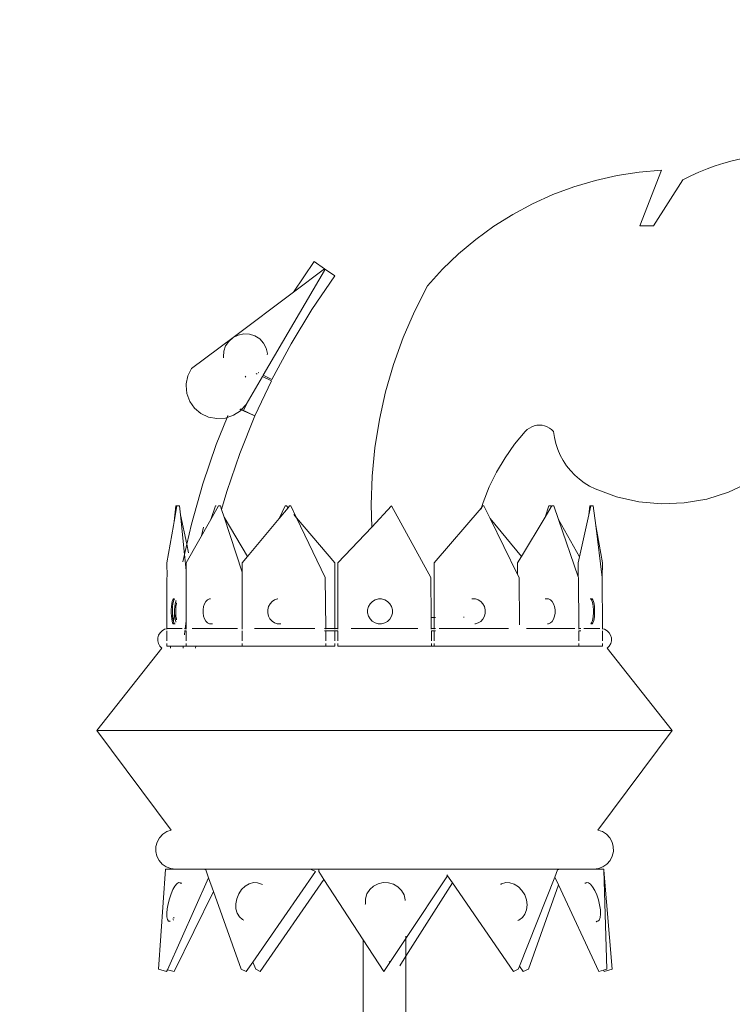
# Model space of a CAD drawing. Units: millimetres. Extents: x 7894 to 8038, y 6851 to 6951.
# Tile 30 of 49: x 7958.696 to 7960.68, y 6925.713 to 6928.453. Entities that reach past the tile are written whole.
import ezdxf

# ---------------------------------------------------------------- set-up
doc = ezdxf.new("R2010")
doc.units = ezdxf.units.MM
doc.layers.add('A-ANNO-DIMS', color=2, linetype='Continuous', lineweight=18)
doc.layers.add('A-FURN-ACCS', color=8, linetype='Continuous', lineweight=13)
doc.styles.get("Standard").update_dxf_attribs({"font": 'arial.ttf'})
doc.dimstyles.new('ISO-25', dxfattribs={"dimtxt": 1, "dimasz": 1, "dimexe": 1.25, "dimexo": 0.625, "dimtad": 1, "dimdec": 0, "dimlunit": 4, "dimtxsty": 'Standard', "dimcen": 2.5, "dimclrt": 1, "dimadec": 0, "dimazin": 0, "dimtfac": 1, "dimtdec": 0, "dimtmove": 0, "dimatfit": 3, "dimfxl": 1, "dimarcsym": 0})

# ---------------------------------------------------------------- blocks, each defined once
blk = doc.blocks.new('DISPLAY-LEAF-FINIAL-Z2_152')
for p, q in [((1.7688, 3.2049, 2.1518), (1.7926, 3.2108, 2.1518)), ((1.5102, 3.1734, 2.1518), (1.5723, 3.1787, 2.1518)), ((1.5723, 3.1787, 2.1518), (1.5113, 3.0242, 2.1518)), ((1.6762, 3.1731, 2.1518), (1.6989, 3.1823, 2.1518)), ((1.6989, 3.1823, 2.1518), (1.7219, 3.1906, 2.1518)), ((1.7219, 3.1906, 2.1518), (1.7452, 3.1982, 2.1518)), ((1.7452, 3.1982, 2.1518), (1.7688, 3.2049, 2.1518)), ((1.3879, 3.1503, 2.1518), (1.4486, 3.1639, 2.1518)), ((1.4486, 3.1639, 2.1518), (1.5102, 3.1734, 2.1518)), ((1.5498, 3.0242, 2.1518), (1.6318, 3.1522, 2.1518)), ((1.6318, 3.1522, 2.1518), (1.6538, 3.163, 2.1518)), ((1.6538, 3.163, 2.1518), (1.6762, 3.1731, 2.1518)), ((1.2698, 3.1109, 2.1518), (1.3281, 3.1326, 2.1518)), ((1.3281, 3.1326, 2.1518), (1.3879, 3.1503, 2.1518)), ((1.213, 3.0852, 2.1518), (1.2698, 3.1109, 2.1518)), ((1.1581, 3.0558, 2.1518), (1.213, 3.0852, 2.1518)), ((1.1053, 3.0227, 2.1518), (1.1581, 3.0558, 2.1518)), ((1.0549, 2.9861, 2.1518), (1.1053, 3.0227, 2.1518)), ((1.5113, 3.0242, 2.1518), (1.5498, 3.0242, 2.1518)), ((1.0071, 2.9462, 2.1518), (1.0549, 2.9861, 2.1518)), ((0.9621, 2.9031, 2.1518), (1.0071, 2.9462, 2.1518)), ((0.6052, 2.9244, 2.1518), (0.5471, 2.8395, 2.1518)), ((0.634, 2.9046, 2.1518), (0.5471, 2.8395, 2.1518)), ((0.634, 2.9046, 2.1518), (0.6052, 2.9244, 2.1518)), ((0.634, 2.9001, 2.1518), (0.634, 2.9046, 2.1518)), ((0.6629, 2.8848, 2.1518), (0.634, 2.9046, 2.1518)), ((0.634, 2.9001, 2.1518), (0.4632, 2.6089, 2.1518)), ((0.5989, 2.7915, 2.1518), (0.6629, 2.8848, 2.1518)), ((0.9202, 2.857, 2.1518), (0.9621, 2.9031, 2.1518)), ((0.9202, 2.857, 2.1518), (0.8844, 2.7861, 2.1518)), ((0.5471, 2.8395, 2.1518), (0.379, 2.7129, 2.1518)), ((0.5406, 2.6956, 2.1518), (0.5989, 2.7915, 2.1518)), ((0.8844, 2.7861, 2.1518), (0.8529, 2.7132, 2.1518)), ((0.379, 2.7129, 2.1518), (0.2637, 2.6275, 2.1518)), ((0.3671, 2.7026, 2.1518), (0.379, 2.7129, 2.1518)), ((0.379, 2.7129, 2.1518), (0.3932, 2.7199, 2.1518)), ((0.3932, 2.7199, 2.1518), (0.4088, 2.7231, 2.1518)), ((0.4088, 2.7231, 2.1518), (0.4248, 2.7223, 2.1518)), ((0.4248, 2.7223, 2.1518), (0.44, 2.7176, 2.1518)), ((0.44, 2.7176, 2.1518), (0.4533, 2.7092, 2.1518)), ((0.8529, 2.7132, 2.1518), (0.8261, 2.6384, 2.1518)), ((0.3535, 2.675, 2.1518), (0.3584, 2.6897, 2.1518)), ((0.3584, 2.6897, 2.1518), (0.3671, 2.7026, 2.1518)), ((0.4533, 2.7092, 2.1518), (0.464, 2.6977, 2.1518)), ((0.464, 2.6977, 2.1518), (0.4713, 2.6839, 2.1518)), ((0.5406, 2.6956, 2.1518), (0.4875, 2.5967, 2.1518)), ((0.3526, 2.6596, 2.1518), (0.3535, 2.675, 2.1518)), ((0.3527, 2.6591, 2.1518), (0.3526, 2.6596, 2.1518)), ((0.3526, 2.6569, 2.1518), (0.3527, 2.6591, 2.1518)), ((0.4713, 2.6839, 2.1518), (0.4746, 2.6689, 2.1518)), ((0.4745, 2.6667, 2.1518), (0.4746, 2.6689, 2.1518)), ((0.4745, 2.6667, 2.1518), (0.4746, 2.6661, 2.1518)), ((0.8261, 2.6384, 2.1518), (0.804, 2.5622, 2.1518)), ((0.2535, 2.6069, 2.1518), (0.249, 2.5845, 2.1518)), ((0.2637, 2.6275, 2.1518), (0.2535, 2.6069, 2.1518)), ((0.4144, 2.6055, 2.1518), (0.4132, 2.6029, 2.1518)), ((0.4608, 2.6047, 2.1518), (0.4152, 2.527, 2.1518)), ((0.4431, 2.613, 2.1518), (0.4459, 2.6117, 2.1518)), ((0.4508, 2.6151, 2.1518), (0.4489, 2.6161, 2.1518)), ((0.4632, 2.6089, 2.1518), (0.4608, 2.6047, 2.1518)), ((0.4858, 2.593, 2.1518), (0.4608, 2.6047, 2.1518)), ((0.4632, 2.6089, 2.1518), (0.4875, 2.5967, 2.1518)), ((0.249, 2.58, 2.1518), (0.249, 2.5845, 2.1518)), ((0.249, 2.58, 2.1518), (0.2508, 2.5572, 2.1518)), ((0.4402, 2.4957, 2.1518), (0.4858, 2.593, 2.1518)), ((0.2508, 2.5572, 2.1518), (0.2586, 2.5356, 2.1518)), ((0.804, 2.5622, 2.1518), (0.7865, 2.4847, 2.1518)), ((0.2586, 2.5356, 2.1518), (0.2719, 2.5167, 2.1518)), ((0.4029, 2.5132, 2.1518), (0.4152, 2.527, 2.1518)), ((0.4202, 2.5355, 2.1518), (0.4085, 2.5106, 2.1518)), ((0.2719, 2.5167, 2.1518), (0.2898, 2.5018, 2.1518)), ((0.2898, 2.5018, 2.1518), (0.3111, 2.4919, 2.1518)), ((0.3628, 2.4909, 2.1518), (0.3802, 2.4968, 2.1518)), ((0.3649, 2.4962, 2.1518), (0.3628, 2.4909, 2.1518)), ((0.3802, 2.4968, 2.1518), (0.3998, 2.5097, 2.1518)), ((0.3978, 2.391, 2.1518), (0.4399, 2.4951, 2.1518)), ((0.3983, 2.5132, 2.1518), (0.4016, 2.5117, 2.1518)), ((0.3998, 2.5097, 2.1518), (0.4016, 2.5117, 2.1518)), ((0.4029, 2.5132, 2.1518), (0.4003, 2.5144, 2.1518)), ((0.4016, 2.5117, 2.1518), (0.4029, 2.5132, 2.1518)), ((0.4016, 2.5117, 2.1518), (0.4399, 2.4951, 2.1518)), ((0.4029, 2.5132, 2.1518), (0.4402, 2.4957, 2.1518)), ((0.4085, 2.5106, 2.1518), (0.4078, 2.509, 2.1518)), ((0.3111, 2.4919, 2.1518), (0.3343, 2.4876, 2.1518)), ((0.3628, 2.4909, 2.1518), (0.3323, 2.4155, 2.1518)), ((0.3343, 2.4876, 2.1518), (0.3579, 2.4893, 2.1518)), ((0.3579, 2.4893, 2.1518), (0.3628, 2.4909, 2.1518)), ((0.7865, 2.4847, 2.1518), (0.774, 2.4062, 2.1518)), ((1.2175, 2.4675, 2.1518), (1.2106, 2.465, 2.1518)), ((1.2247, 2.469, 2.1518), (1.2175, 2.4675, 2.1518)), ((1.2321, 2.4695, 2.1518), (1.2247, 2.469, 2.1518)), ((1.2395, 2.469, 2.1518), (1.2321, 2.4695, 2.1518)), ((1.2467, 2.4675, 2.1518), (1.2395, 2.469, 2.1518)), ((1.2536, 2.465, 2.1518), (1.2467, 2.4675, 2.1518)), ((1.1928, 2.4521, 2.1518), (1.1631, 2.4165, 2.1518)), ((1.1981, 2.4572, 2.1518), (1.1928, 2.4521, 2.1518)), ((1.2041, 2.4615, 2.1518), (1.1981, 2.4572, 2.1518)), ((1.2106, 2.465, 2.1518), (1.2041, 2.4615, 2.1518)), ((1.2601, 2.4615, 2.1518), (1.2536, 2.465, 2.1518)), ((1.2661, 2.4572, 2.1518), (1.2601, 2.4615, 2.1518)), ((1.2714, 2.4521, 2.1518), (1.2661, 2.4572, 2.1518)), ((1.274, 2.435, 2.1518), (1.2714, 2.4521, 2.1518)), ((0.3323, 2.4155, 2.1518), (0.2946, 2.3057, 2.1518)), ((1.1631, 2.4165, 2.1518), (1.1364, 2.3788, 2.1518)), ((1.278, 2.4183, 2.1518), (1.274, 2.435, 2.1518)), ((1.2834, 2.4019, 2.1518), (1.278, 2.4183, 2.1518)), ((0.3614, 2.2848, 2.1518), (0.3978, 2.391, 2.1518)), ((0.774, 2.4062, 2.1518), (0.7662, 2.3272, 2.1518)), ((1.2903, 2.3861, 2.1518), (1.2834, 2.4019, 2.1518)), ((1.2985, 2.371, 2.1518), (1.2903, 2.3861, 2.1518)), ((1.1364, 2.3788, 2.1518), (1.1127, 2.339, 2.1518)), ((1.308, 2.3566, 2.1518), (1.2985, 2.371, 2.1518)), ((1.3187, 2.3431, 2.1518), (1.308, 2.3566, 2.1518)), ((1.1127, 2.339, 2.1518), (1.0923, 2.2975, 2.1518)), ((1.3305, 2.3306, 2.1518), (1.3187, 2.3431, 2.1518)), ((1.3434, 2.3192, 2.1518), (1.3305, 2.3306, 2.1518)), ((0.2946, 2.3057, 2.1518), (0.263, 2.1941, 2.1518)), ((0.7662, 2.3272, 2.1518), (0.7634, 2.2478, 2.1518)), ((1.3572, 2.3089, 2.1518), (1.3434, 2.3192, 2.1518)), ((1.3719, 2.2999, 2.1518), (1.3572, 2.3089, 2.1518)), ((1.8161, 2.3099, 2.1518), (1.7585, 2.283, 2.1518)), ((0.3472, 2.2349, 2.1518), (0.3614, 2.2848, 2.1518)), ((1.0923, 2.2975, 2.1518), (1.0752, 2.2545, 2.1518)), ((1.3873, 2.2921, 2.1518), (1.3719, 2.2999, 2.1518)), ((1.4468, 2.2701, 2.1518), (1.3873, 2.2921, 2.1518)), ((1.7585, 2.283, 2.1518), (1.698, 2.2639, 2.1518)), ((0.7634, 2.2478, 2.1518), (0.7651, 2.1857, 2.1518)), ((1.0752, 2.2545, 2.1518), (1.0707, 2.2401, 2.1518)), ((1.5088, 2.256, 2.1518), (1.4468, 2.2701, 2.1518)), ((1.572, 2.2503, 2.1518), (1.5088, 2.256, 2.1518)), ((1.6354, 2.2529, 2.1518), (1.572, 2.2503, 2.1518)), ((1.698, 2.2639, 2.1518), (1.6354, 2.2529, 2.1518)), ((0.2147, 2.201, 2.1518), (0.2202, 2.2445, 2.1518)), ((0.223, 2.2445, 2.1518), (0.2147, 2.201, 2.1518)), ((0.223, 2.2445, 2.1518), (0.2202, 2.2445, 2.1518)), ((0.223, 2.2445, 2.1518), (0.2299, 2.2445, 2.1518)), ((0.2325, 2.2195, 2.1518), (0.2299, 2.2445, 2.1518)), ((0.2325, 2.2195, 2.1518), (0.2504, 2.1381, 2.1518)), ((0.2439, 2.1095, 2.1518), (0.2325, 2.2195, 2.1518)), ((0.3171, 2.2068, 2.1518), (0.3302, 2.2445, 2.1518)), ((0.3384, 2.2445, 2.1518), (0.3171, 2.2068, 2.1518)), ((0.3318, 2.2445, 2.1518), (0.3302, 2.2445, 2.1518)), ((0.344, 2.2445, 2.1518), (0.3384, 2.2445, 2.1518)), ((0.3472, 2.2349, 2.1518), (0.344, 2.2445, 2.1518)), ((0.3543, 2.2133, 2.1518), (0.3472, 2.2349, 2.1518)), ((0.5072, 2.2093, 2.1518), (0.5246, 2.2445, 2.1518)), ((0.5322, 2.2392, 2.1518), (0.5072, 2.2093, 2.1518)), ((0.5277, 2.2445, 2.1518), (0.5246, 2.2445, 2.1518)), ((0.5277, 2.2445, 2.1518), (0.5322, 2.2392, 2.1518)), ((0.5366, 2.2445, 2.1518), (0.5322, 2.2392, 2.1518)), ((0.5399, 2.2445, 2.1518), (0.5366, 2.2445, 2.1518)), ((0.5559, 2.2114, 2.1518), (0.5399, 2.2445, 2.1518)), ((0.5482, 2.2204, 2.1518), (0.5559, 2.2114, 2.1518)), ((0.8207, 2.2445, 2.1518), (0.7651, 2.1857, 2.1518)), ((0.93, 2.0453, 2.1518), (0.8207, 2.2445, 2.1518)), ((1.0703, 2.2388, 2.1518), (0.9393, 2.0859, 2.1518)), ((1.0703, 2.2388, 2.1518), (1.069, 2.2345, 2.1518)), ((1.0707, 2.2401, 2.1518), (1.0703, 2.2388, 2.1518)), ((1.0703, 2.2388, 2.1518), (1.0715, 2.2374, 2.1518)), ((1.0745, 2.2445, 2.1518), (1.0707, 2.2401, 2.1518)), ((1.0745, 2.2445, 2.1518), (1.0775, 2.2445, 2.1518)), ((1.0949, 2.2093, 2.1518), (1.0775, 2.2445, 2.1518)), ((1.2478, 2.2133, 2.1518), (1.2581, 2.2445, 2.1518)), ((1.2651, 2.2421, 2.1518), (1.2478, 2.2133, 2.1518)), ((1.2581, 2.2445, 2.1518), (1.2637, 2.2445, 2.1518)), ((1.2637, 2.2445, 2.1518), (1.2651, 2.2421, 2.1518)), ((1.2666, 2.2445, 2.1518), (1.2651, 2.2421, 2.1518)), ((1.2666, 2.2445, 2.1518), (1.272, 2.2445, 2.1518)), ((1.2851, 2.2068, 2.1518), (1.272, 2.2445, 2.1518)), ((1.3696, 2.2195, 2.1518), (1.344, 2.1028, 2.1518)), ((1.3696, 2.2195, 2.1518), (1.3722, 2.2445, 2.1518)), ((1.3751, 2.2445, 2.1518), (1.3696, 2.2195, 2.1518)), ((1.3722, 2.2445, 2.1518), (1.3751, 2.2445, 2.1518)), ((1.3751, 2.2445, 2.1518), (1.3819, 2.2445, 2.1518)), ((1.3819, 2.2445, 2.1518), (1.3889, 2.1901, 2.1518)), ((0.2133, 2.1901, 2.1518), (0.2147, 2.201, 2.1518)), ((0.3171, 2.2068, 2.1518), (0.2485, 2.0859, 2.1518)), ((0.263, 2.1941, 2.1518), (0.2504, 2.1381, 2.1518)), ((0.3543, 2.2133, 2.1518), (0.4197, 2.1042, 2.1518)), ((0.4044, 2.0607, 2.1518), (0.3543, 2.2133, 2.1518)), ((0.5072, 2.2093, 2.1518), (0.4197, 2.1042, 2.1518)), ((0.5559, 2.2114, 2.1518), (0.6628, 2.0859, 2.1518)), ((0.636, 2.0453, 2.1518), (0.5559, 2.2114, 2.1518)), ((1.0949, 2.2093, 2.1518), (1.1824, 2.1042, 2.1518)), ((1.0949, 2.2093, 2.1518), (1.1714, 2.0542, 2.1518)), ((1.2478, 2.2133, 2.1518), (1.1824, 2.1042, 2.1518)), ((1.2851, 2.2068, 2.1518), (1.344, 2.1028, 2.1518)), ((1.2851, 2.2068, 2.1518), (1.3403, 2.0478, 2.1518)), ((0.2133, 2.1901, 2.1518), (0.1946, 2.0859, 2.1518)), ((0.2969, 2.1855, 2.1518), (0.2915, 2.1618, 2.1518)), ((0.7651, 2.1857, 2.1518), (0.6705, 2.0859, 2.1518)), ((1.3889, 2.1901, 2.1518), (1.4075, 2.0859, 2.1518)), ((1.4073, 2.0453, 2.1518), (1.3889, 2.1901, 2.1518)), ((0.2504, 2.1381, 2.1518), (0.2439, 2.1095, 2.1518)), ((0.2504, 2.1381, 2.1518), (0.2555, 2.1145, 2.1518)), ((0.1946, 2.0859, 2.1518), (0.1952, 2.0478, 2.1518)), ((0.2439, 2.1095, 2.1518), (0.2392, 2.0887, 2.1518)), ((0.2485, 2.0654, 2.1518), (0.2439, 2.1095, 2.1518)), ((0.2485, 2.0859, 2.1518), (0.2485, 2.0654, 2.1518)), ((0.4197, 2.1042, 2.1518), (0.4044, 2.0859, 2.1518)), ((0.4044, 2.0859, 2.1518), (0.4044, 2.0607, 2.1518)), ((0.6628, 2.0859, 2.1518), (0.6628, 1.9035, 2.1518)), ((0.6705, 2.0859, 2.1518), (0.6705, 1.9035, 2.1518)), ((0.9393, 2.0859, 2.1518), (0.9393, 1.9343, 2.1518)), ((1.1824, 2.1042, 2.1518), (1.1714, 2.0859, 2.1518)), ((1.1714, 2.0859, 2.1518), (1.1714, 2.0542, 2.1518)), ((1.344, 2.1028, 2.1518), (1.3403, 2.0859, 2.1518)), ((1.3403, 2.0859, 2.1518), (1.3403, 2.0478, 2.1518)), ((1.4075, 2.0859, 2.1518), (1.4073, 2.0453, 2.1518)), ((0.2485, 2.0654, 2.1518), (0.2485, 1.9035, 2.1518)), ((0.4044, 2.0607, 2.1518), (0.4044, 1.9015, 2.1518)), ((0.1949, 2.0453, 2.1518), (0.1946, 1.903, 2.1518)), ((0.1949, 2.0453, 2.1518), (0.1952, 2.0478, 2.1518)), ((0.636, 2.0453, 2.1518), (0.6371, 1.9035, 2.1518)), ((0.93, 2.0453, 2.1518), (0.9309, 1.9342, 2.1518)), ((1.1758, 2.0453, 2.1518), (1.1714, 2.0542, 2.1518)), ((1.1758, 2.0453, 2.1518), (1.1768, 1.9142, 2.1518)), ((1.3412, 2.0453, 2.1518), (1.3403, 2.0478, 2.1518)), ((1.3412, 2.0453, 2.1518), (1.3419, 1.9035, 2.1518)), ((1.4073, 2.0453, 2.1518), (1.4075, 1.903, 2.1518)), ((0.2074, 1.9648, 2.1518), (0.2082, 1.9727, 2.1518)), ((0.2082, 1.9727, 2.1518), (0.2095, 1.9791, 2.1518)), ((0.2095, 1.9791, 2.1518), (0.211, 1.9837, 2.1518)), ((0.2108, 1.9648, 2.1518), (0.2117, 1.9727, 2.1518)), ((0.211, 1.9837, 2.1518), (0.2126, 1.986, 2.1518)), ((0.2117, 1.9727, 2.1518), (0.2129, 1.9791, 2.1518)), ((0.2161, 1.986, 2.1518), (0.2126, 1.986, 2.1518)), ((0.2129, 1.9791, 2.1518), (0.2144, 1.9837, 2.1518)), ((0.2144, 1.9837, 2.1518), (0.2161, 1.986, 2.1518)), ((0.2194, 1.979, 2.1518), (0.2179, 1.9725, 2.1518)), ((0.2202, 1.9812, 2.1518), (0.2194, 1.979, 2.1518)), ((0.2204, 1.9806, 2.1518), (0.2194, 1.979, 2.1518)), ((0.2218, 1.9746, 2.1518), (0.2213, 1.9725, 2.1518)), ((0.2969, 1.9648, 2.1518), (0.2996, 1.9727, 2.1518)), ((0.2996, 1.9727, 2.1518), (0.3035, 1.9791, 2.1518)), ((0.3035, 1.9791, 2.1518), (0.3083, 1.9837, 2.1518)), ((0.3083, 1.9837, 2.1518), (0.3135, 1.986, 2.1518)), ((0.3163, 1.986, 2.1518), (0.3135, 1.986, 2.1518)), ((0.478, 1.9648, 2.1518), (0.482, 1.9727, 2.1518)), ((0.482, 1.9727, 2.1518), (0.4877, 1.9791, 2.1518)), ((0.4877, 1.9791, 2.1518), (0.4947, 1.9837, 2.1518)), ((0.4947, 1.9837, 2.1518), (0.5025, 1.986, 2.1518)), ((0.5041, 1.986, 2.1518), (0.5025, 1.986, 2.1518)), ((0.756, 1.9648, 2.1518), (0.7606, 1.9727, 2.1518)), ((0.7606, 1.9727, 2.1518), (0.7671, 1.9791, 2.1518)), ((0.7671, 1.9791, 2.1518), (0.775, 1.9837, 2.1518)), ((0.775, 1.9837, 2.1518), (0.7838, 1.986, 2.1518)), ((0.7838, 1.986, 2.1518), (0.7929, 1.986, 2.1518)), ((0.7929, 1.986, 2.1518), (0.8018, 1.9836, 2.1518)), ((0.8018, 1.9836, 2.1518), (0.8096, 1.979, 2.1518)), ((0.8096, 1.979, 2.1518), (0.8161, 1.9725, 2.1518)), ((1.0443, 1.986, 2.1518), (1.0459, 1.986, 2.1518)), ((1.0459, 1.986, 2.1518), (1.0541, 1.986, 2.1518)), ((1.0541, 1.986, 2.1518), (1.062, 1.9836, 2.1518)), ((1.062, 1.9836, 2.1518), (1.0691, 1.979, 2.1518)), ((1.0691, 1.979, 2.1518), (1.0749, 1.9725, 2.1518)), ((1.2486, 1.986, 2.1518), (1.2513, 1.986, 2.1518)), ((1.2513, 1.986, 2.1518), (1.2571, 1.986, 2.1518)), ((1.2571, 1.986, 2.1518), (1.2627, 1.9836, 2.1518)), ((1.2627, 1.9836, 2.1518), (1.2677, 1.979, 2.1518)), ((1.2677, 1.979, 2.1518), (1.2717, 1.9725, 2.1518)), ((1.3734, 1.986, 2.1518), (1.3755, 1.986, 2.1518)), ((1.3755, 1.986, 2.1518), (1.3775, 1.9836, 2.1518)), ((1.3755, 1.986, 2.1518), (1.3768, 1.986, 2.1518)), ((1.3768, 1.986, 2.1518), (1.3789, 1.986, 2.1518)), ((1.3775, 1.9836, 2.1518), (1.3794, 1.979, 2.1518)), ((1.3789, 1.986, 2.1518), (1.3809, 1.9836, 2.1518)), ((1.3794, 1.979, 2.1518), (1.3809, 1.9725, 2.1518)), ((1.3809, 1.9836, 2.1518), (1.3828, 1.979, 2.1518)), ((1.3828, 1.979, 2.1518), (1.3843, 1.9725, 2.1518)), ((0.2069, 1.956, 2.1518), (0.2074, 1.9648, 2.1518)), ((0.2069, 1.9469, 2.1518), (0.2069, 1.956, 2.1518)), ((0.2073, 1.938, 2.1518), (0.2069, 1.9469, 2.1518)), ((0.2103, 1.956, 2.1518), (0.2108, 1.9648, 2.1518)), ((0.2103, 1.9469, 2.1518), (0.2103, 1.956, 2.1518)), ((0.2108, 1.938, 2.1518), (0.2103, 1.9469, 2.1518)), ((0.2163, 1.9467, 2.1518), (0.2129, 1.9237, 2.1518)), ((0.2168, 1.9646, 2.1518), (0.2163, 1.9558, 2.1518)), ((0.2163, 1.9558, 2.1518), (0.2163, 1.9467, 2.1518)), ((0.2163, 1.9467, 2.1518), (0.2168, 1.9379, 2.1518)), ((0.2179, 1.9725, 2.1518), (0.2168, 1.9646, 2.1518)), ((0.218, 1.9665, 2.1518), (0.2168, 1.9646, 2.1518)), ((0.2179, 1.9725, 2.1518), (0.218, 1.9665, 2.1518)), ((0.2202, 1.9646, 2.1518), (0.2197, 1.9558, 2.1518)), ((0.2197, 1.9558, 2.1518), (0.2197, 1.9467, 2.1518)), ((0.2197, 1.9467, 2.1518), (0.2202, 1.9379, 2.1518)), ((0.2213, 1.9725, 2.1518), (0.2202, 1.9646, 2.1518)), ((0.2955, 1.956, 2.1518), (0.2969, 1.9648, 2.1518)), ((0.2955, 1.9469, 2.1518), (0.2955, 1.956, 2.1518)), ((0.2969, 1.938, 2.1518), (0.2955, 1.9469, 2.1518)), ((0.4759, 1.956, 2.1518), (0.478, 1.9648, 2.1518)), ((0.4759, 1.9469, 2.1518), (0.4759, 1.956, 2.1518)), ((0.4779, 1.938, 2.1518), (0.4759, 1.9469, 2.1518)), ((0.7536, 1.956, 2.1518), (0.756, 1.9648, 2.1518)), ((0.7536, 1.9469, 2.1518), (0.7536, 1.956, 2.1518)), ((0.756, 1.938, 2.1518), (0.7536, 1.9469, 2.1518)), ((0.8161, 1.9725, 2.1518), (0.8206, 1.9646, 2.1518)), ((0.8229, 1.9467, 2.1518), (0.8205, 1.9379, 2.1518)), ((0.8206, 1.9646, 2.1518), (0.823, 1.9558, 2.1518)), ((0.823, 1.9558, 2.1518), (0.8229, 1.9467, 2.1518)), ((1.0749, 1.9725, 2.1518), (1.079, 1.9646, 2.1518)), ((1.081, 1.9467, 2.1518), (1.0789, 1.9379, 2.1518)), ((1.079, 1.9646, 2.1518), (1.0811, 1.9558, 2.1518)), ((1.0811, 1.9558, 2.1518), (1.081, 1.9467, 2.1518)), ((1.2717, 1.9725, 2.1518), (1.2746, 1.9646, 2.1518)), ((1.2746, 1.9646, 2.1518), (1.2761, 1.9558, 2.1518)), ((1.2761, 1.9467, 2.1518), (1.2746, 1.9379, 2.1518)), ((1.2761, 1.9558, 2.1518), (1.2761, 1.9467, 2.1518)), ((1.3809, 1.9725, 2.1518), (1.3819, 1.9646, 2.1518)), ((1.3819, 1.9646, 2.1518), (1.3825, 1.9558, 2.1518)), ((1.3824, 1.9467, 2.1518), (1.3819, 1.9379, 2.1518)), ((1.3825, 1.9558, 2.1518), (1.3824, 1.9467, 2.1518)), ((1.3843, 1.9725, 2.1518), (1.3853, 1.9646, 2.1518)), ((1.3853, 1.9646, 2.1518), (1.3859, 1.9558, 2.1518)), ((1.3858, 1.9467, 2.1518), (1.3853, 1.9379, 2.1518)), ((1.3859, 1.9558, 2.1518), (1.3858, 1.9467, 2.1518)), ((0.2082, 1.9301, 2.1518), (0.2073, 1.938, 2.1518)), ((0.2094, 1.9237, 2.1518), (0.2082, 1.9301, 2.1518)), ((0.2109, 1.9191, 2.1518), (0.2094, 1.9237, 2.1518)), ((0.2116, 1.9301, 2.1518), (0.2108, 1.938, 2.1518)), ((0.2126, 1.9167, 2.1518), (0.2109, 1.9191, 2.1518)), ((0.2129, 1.9237, 2.1518), (0.2116, 1.9301, 2.1518)), ((0.2143, 1.9191, 2.1518), (0.2129, 1.9237, 2.1518)), ((0.216, 1.9167, 2.1518), (0.2143, 1.9191, 2.1518)), ((0.2168, 1.9379, 2.1518), (0.2179, 1.93, 2.1518)), ((0.2179, 1.93, 2.1518), (0.2194, 1.9235, 2.1518)), ((0.2194, 1.9235, 2.1518), (0.2202, 1.9215, 2.1518)), ((0.2202, 1.9379, 2.1518), (0.2213, 1.93, 2.1518)), ((0.2213, 1.93, 2.1518), (0.2218, 1.928, 2.1518)), ((0.2485, 1.9251, 2.1518), (0.2458, 1.9015, 2.1518)), ((0.2996, 1.9301, 2.1518), (0.2969, 1.938, 2.1518)), ((0.3034, 1.9237, 2.1518), (0.2996, 1.9301, 2.1518)), ((0.3082, 1.9191, 2.1518), (0.3034, 1.9237, 2.1518)), ((0.3134, 1.9167, 2.1518), (0.3082, 1.9191, 2.1518)), ((0.4819, 1.9301, 2.1518), (0.4779, 1.938, 2.1518)), ((0.4876, 1.9237, 2.1518), (0.4819, 1.9301, 2.1518)), ((0.4945, 1.9191, 2.1518), (0.4876, 1.9237, 2.1518)), ((0.5023, 1.9167, 2.1518), (0.4945, 1.9191, 2.1518)), ((0.7605, 1.9301, 2.1518), (0.756, 1.938, 2.1518)), ((0.7669, 1.9237, 2.1518), (0.7605, 1.9301, 2.1518)), ((0.7748, 1.9191, 2.1518), (0.7669, 1.9237, 2.1518)), ((0.7836, 1.9167, 2.1518), (0.7748, 1.9191, 2.1518)), ((0.8016, 1.919, 2.1518), (0.7928, 1.9167, 2.1518)), ((0.8095, 1.9235, 2.1518), (0.8016, 1.919, 2.1518)), ((0.816, 1.93, 2.1518), (0.8095, 1.9235, 2.1518)), ((0.8205, 1.9379, 2.1518), (0.816, 1.93, 2.1518)), ((0.9393, 1.9343, 2.1518), (0.9309, 1.9342, 2.1518)), ((0.9309, 1.9342, 2.1518), (0.9312, 1.9035, 2.1518)), ((0.9424, 1.9343, 2.1518), (0.9393, 1.9343, 2.1518)), ((0.9393, 1.9343, 2.1518), (0.9393, 1.9035, 2.1518)), ((1.0224, 1.935, 2.1518), (1.0208, 1.935, 2.1518)), ((1.0618, 1.919, 2.1518), (1.0539, 1.9167, 2.1518)), ((1.069, 1.9235, 2.1518), (1.0618, 1.919, 2.1518)), ((1.0748, 1.93, 2.1518), (1.069, 1.9235, 2.1518)), ((1.0789, 1.9379, 2.1518), (1.0748, 1.93, 2.1518)), ((1.2626, 1.919, 2.1518), (1.257, 1.9167, 2.1518)), ((1.2676, 1.9235, 2.1518), (1.2626, 1.919, 2.1518)), ((1.2717, 1.93, 2.1518), (1.2676, 1.9235, 2.1518)), ((1.2746, 1.9379, 2.1518), (1.2717, 1.93, 2.1518)), ((1.3775, 1.919, 2.1518), (1.3755, 1.9167, 2.1518)), ((1.3793, 1.9235, 2.1518), (1.3775, 1.919, 2.1518)), ((1.3809, 1.919, 2.1518), (1.3789, 1.9167, 2.1518)), ((1.3808, 1.93, 2.1518), (1.3793, 1.9235, 2.1518)), ((1.3819, 1.9379, 2.1518), (1.3808, 1.93, 2.1518)), ((1.3827, 1.9235, 2.1518), (1.3809, 1.919, 2.1518)), ((1.3842, 1.93, 2.1518), (1.3827, 1.9235, 2.1518)), ((1.3853, 1.9379, 2.1518), (1.3842, 1.93, 2.1518)), ((0.1719, 1.8852, 2.1518), (0.1759, 1.892, 2.1518)), ((0.1759, 1.892, 2.1518), (0.1817, 1.8976, 2.1518)), ((0.1817, 1.8976, 2.1518), (0.1886, 1.9015, 2.1518)), ((0.1886, 1.9015, 2.1518), (0.1946, 1.903, 2.1518)), ((0.1946, 1.8976, 2.1518), (0.1945, 1.8695, 2.1518)), ((0.1946, 1.903, 2.1518), (0.1964, 1.9035, 2.1518)), ((0.1946, 1.903, 2.1518), (0.1946, 1.9015, 2.1518)), ((0.1964, 1.9035, 2.1518), (0.1977, 1.9034, 2.1518)), ((0.1964, 1.9035, 2.1518), (0.1969, 1.9035, 2.1518)), ((0.2373, 1.9035, 2.1518), (0.1977, 1.9034, 2.1518)), ((0.2143, 1.9167, 2.1518), (0.2126, 1.9167, 2.1518)), ((0.216, 1.9167, 2.1518), (0.2143, 1.9167, 2.1518)), ((0.2177, 1.9167, 2.1518), (0.216, 1.9167, 2.1518)), ((0.2485, 1.9035, 2.1518), (0.2439, 1.9035, 2.1518)), ((0.2453, 1.8976, 2.1518), (0.2439, 1.8856, 2.1518)), ((0.2485, 1.8971, 2.1518), (0.2439, 1.8971, 2.1518)), ((0.2485, 1.9035, 2.1518), (0.2485, 1.9015, 2.1518)), ((0.2485, 1.8976, 2.1518), (0.2485, 1.8971, 2.1518)), ((0.2485, 1.8971, 2.1518), (0.2485, 1.8695, 2.1518)), ((0.3912, 1.9035, 2.1518), (0.265, 1.9035, 2.1518)), ((0.3189, 1.9167, 2.1518), (0.3134, 1.9167, 2.1518)), ((0.3217, 1.9167, 2.1518), (0.3189, 1.9167, 2.1518)), ((0.4044, 1.8976, 2.1518), (0.4044, 1.8695, 2.1518)), ((0.4385, 1.9035, 2.1518), (0.6066, 1.9035, 2.1518)), ((0.5103, 1.9167, 2.1518), (0.5023, 1.9167, 2.1518)), ((0.512, 1.9167, 2.1518), (0.5103, 1.9167, 2.1518)), ((0.6371, 1.9035, 2.1518), (0.6338, 1.9035, 2.1518)), ((0.6371, 1.8971, 2.1518), (0.6338, 1.8971, 2.1518)), ((0.6371, 1.9035, 2.1518), (0.6371, 1.9015, 2.1518)), ((0.6628, 1.9035, 2.1518), (0.6371, 1.9035, 2.1518)), ((0.6371, 1.8976, 2.1518), (0.6371, 1.8971, 2.1518)), ((0.6371, 1.8971, 2.1518), (0.6373, 1.8695, 2.1518)), ((0.6628, 1.8971, 2.1518), (0.6371, 1.8971, 2.1518)), ((0.6628, 1.9035, 2.1518), (0.6705, 1.9035, 2.1518)), ((0.6628, 1.9035, 2.1518), (0.6628, 1.9015, 2.1518)), ((0.6628, 1.8976, 2.1518), (0.6628, 1.8971, 2.1518)), ((0.6628, 1.8971, 2.1518), (0.6628, 1.8695, 2.1518)), ((0.6705, 1.8971, 2.1518), (0.6628, 1.8971, 2.1518)), ((0.6705, 1.9035, 2.1518), (0.6705, 1.9015, 2.1518)), ((0.6705, 1.8976, 2.1518), (0.6705, 1.8971, 2.1518)), ((0.6705, 1.8971, 2.1518), (0.6705, 1.8695, 2.1518)), ((0.7081, 1.9035, 2.1518), (0.894, 1.9035, 2.1518)), ((0.7928, 1.9167, 2.1518), (0.7836, 1.9167, 2.1518)), ((0.9312, 1.9035, 2.1518), (0.9312, 1.9015, 2.1518)), ((0.9393, 1.9035, 2.1518), (0.9312, 1.9035, 2.1518)), ((0.9313, 1.8976, 2.1518), (0.9313, 1.8971, 2.1518)), ((0.9313, 1.8971, 2.1518), (0.9315, 1.8695, 2.1518)), ((0.9393, 1.8971, 2.1518), (0.9313, 1.8971, 2.1518)), ((0.9424, 1.9035, 2.1518), (0.9393, 1.9035, 2.1518)), ((0.9393, 1.9035, 2.1518), (0.9393, 1.9015, 2.1518)), ((0.9393, 1.8976, 2.1518), (0.9393, 1.8971, 2.1518)), ((0.9424, 1.8971, 2.1518), (0.9393, 1.8971, 2.1518)), ((0.9393, 1.8971, 2.1518), (0.9393, 1.8695, 2.1518)), ((0.9534, 1.9035, 2.1518), (1.1456, 1.9035, 2.1518)), ((1.0524, 1.9167, 2.1518), (1.0539, 1.9167, 2.1518)), ((1.3304, 1.9035, 2.1518), (1.1965, 1.9035, 2.1518)), ((1.2543, 1.9167, 2.1518), (1.257, 1.9167, 2.1518)), ((1.3471, 1.9035, 2.1518), (1.3419, 1.9035, 2.1518)), ((1.3419, 1.9035, 2.1518), (1.342, 1.9015, 2.1518)), ((1.342, 1.8976, 2.1518), (1.342, 1.8971, 2.1518)), ((1.3471, 1.8971, 2.1518), (1.342, 1.8971, 2.1518)), ((1.342, 1.8971, 2.1518), (1.3421, 1.8695, 2.1518)), ((1.3561, 1.9035, 2.1518), (1.4004, 1.9035, 2.1518)), ((1.3755, 1.9167, 2.1518), (1.3789, 1.9167, 2.1518)), ((1.4075, 1.903, 2.1518), (1.4135, 1.9015, 2.1518)), ((1.4075, 1.903, 2.1518), (1.4075, 1.9015, 2.1518)), ((1.4075, 1.8976, 2.1518), (1.4075, 1.8695, 2.1518)), ((1.4135, 1.9015, 2.1518), (1.4205, 1.8976, 2.1518)), ((1.4205, 1.8976, 2.1518), (1.4262, 1.892, 2.1518)), ((1.4262, 1.892, 2.1518), (1.4303, 1.8852, 2.1518)), ((0.1696, 1.8695, 2.1518), (0.1697, 1.8775, 2.1518)), ((0.1715, 1.8618, 2.1518), (0.1696, 1.8695, 2.1518)), ((0.1697, 1.8775, 2.1518), (0.1719, 1.8852, 2.1518)), ((1.4303, 1.8852, 2.1518), (1.4325, 1.8775, 2.1518)), ((1.4326, 1.8695, 2.1518), (1.4306, 1.8618, 2.1518)), ((1.4325, 1.8775, 2.1518), (1.4326, 1.8695, 2.1518)), ((0, 1.6201, 2.1518), (0.181, 1.8491, 2.1518)), ((0.1754, 1.8548, 2.1518), (0.1715, 1.8618, 2.1518)), ((0.181, 1.8491, 2.1518), (0.1754, 1.8548, 2.1518)), ((0.1945, 1.8618, 2.1518), (0.1945, 1.8548, 2.1518)), ((0.1952, 1.8548, 2.1518), (0.1945, 1.8548, 2.1518)), ((0.2052, 1.8548, 2.1518), (0.1945, 1.8548, 2.1518)), ((0.2048, 1.8513, 2.1518), (0.2047, 1.8491, 2.1518)), ((0.2052, 1.8548, 2.1518), (0.2048, 1.8513, 2.1518)), ((0.2485, 1.8548, 2.1518), (0.2052, 1.8548, 2.1518)), ((0.2404, 1.8548, 2.1518), (0.2398, 1.8491, 2.1518)), ((0.2485, 1.8618, 2.1518), (0.2485, 1.8548, 2.1518)), ((0.2485, 1.8548, 2.1518), (0.2756, 1.8548, 2.1518)), ((0.2749, 1.8491, 2.1518), (0.2756, 1.8548, 2.1518)), ((0.2756, 1.8548, 2.1518), (0.4049, 1.8548, 2.1518)), ((0.4044, 1.8618, 2.1518), (0.4049, 1.8548, 2.1518)), ((0.4049, 1.8548, 2.1518), (0.6375, 1.8548, 2.1518)), ((0.6374, 1.8618, 2.1518), (0.6375, 1.8548, 2.1518)), ((0.6628, 1.8548, 2.1518), (0.6375, 1.8548, 2.1518)), ((0.6628, 1.8618, 2.1518), (0.6628, 1.8548, 2.1518)), ((0.6705, 1.8618, 2.1518), (0.6705, 1.8548, 2.1518)), ((0.6705, 1.8548, 2.1518), (0.9316, 1.8548, 2.1518)), ((0.9316, 1.8618, 2.1518), (0.9316, 1.8548, 2.1518)), ((0.9393, 1.8548, 2.1518), (0.9316, 1.8548, 2.1518)), ((0.9393, 1.8618, 2.1518), (0.9393, 1.8548, 2.1518)), ((1.3422, 1.8548, 2.1518), (0.9393, 1.8548, 2.1518)), ((1.3422, 1.8618, 2.1518), (1.3422, 1.8548, 2.1518)), ((1.4075, 1.8548, 2.1518), (1.3422, 1.8548, 2.1518)), ((1.4075, 1.8618, 2.1518), (1.4075, 1.8548, 2.1518)), ((1.4267, 1.8548, 2.1518), (1.4212, 1.8491, 2.1518)), ((1.4212, 1.8491, 2.1518), (1.6021, 1.6201, 2.1518)), ((1.4306, 1.8618, 2.1518), (1.4267, 1.8548, 2.1518)), ((0.2072, 1.3429, 2.1518), (0, 1.6201, 2.1518)), ((1.6021, 1.6201, 2.1518), (0, 1.6201, 2.1518)), ((1.6021, 1.6201, 2.1518), (1.395, 1.3429, 2.1518)), ((0.1945, 1.3385, 2.1518), (0.2072, 1.3429, 2.1518)), ((1.395, 1.3429, 2.1518), (1.4076, 1.3385, 2.1518)), ((0.1678, 1.3095, 2.1518), (0.1742, 1.3213, 2.1518)), ((0.1742, 1.3213, 2.1518), (0.1833, 1.3311, 2.1518)), ((0.1833, 1.3311, 2.1518), (0.1945, 1.3385, 2.1518)), ((1.4076, 1.3385, 2.1518), (1.4188, 1.3311, 2.1518)), ((1.4188, 1.3311, 2.1518), (1.4279, 1.3213, 2.1518)), ((1.4279, 1.3213, 2.1518), (1.4344, 1.3095, 2.1518)), ((0.1641, 1.2832, 2.1518), (0.1643, 1.2966, 2.1518)), ((0.1643, 1.2966, 2.1518), (0.1678, 1.3095, 2.1518)), ((1.4344, 1.3095, 2.1518), (1.4378, 1.2966, 2.1518)), ((1.4378, 1.2966, 2.1518), (1.438, 1.2832, 2.1518)), ((0.1672, 1.2701, 2.1518), (0.1641, 1.2832, 2.1518)), ((0.1733, 1.2582, 2.1518), (0.1672, 1.2701, 2.1518)), ((1.435, 1.2701, 2.1518), (1.4288, 1.2582, 2.1518)), ((1.438, 1.2832, 2.1518), (1.435, 1.2701, 2.1518)), ((0.1714, 0.9553, 2.1518), (0.1907, 1.234, 2.1518)), ((0.1821, 1.2481, 2.1518), (0.1733, 1.2582, 2.1518)), ((0.1931, 1.2404, 2.1518), (0.1821, 1.2481, 2.1518)), ((0.2189, 1.234, 2.1518), (0.1907, 1.234, 2.1518)), ((0.2056, 1.2356, 2.1518), (0.1931, 1.2404, 2.1518)), ((0.2189, 1.234, 2.1518), (0.2056, 1.2356, 2.1518)), ((0.2189, 1.234, 2.1518), (0.2969, 1.234, 2.1518)), ((0.2969, 1.234, 2.1518), (0.3022, 1.234, 2.1518)), ((0.3029, 1.2321, 2.1518), (0.2969, 1.234, 2.1518)), ((0.3029, 1.2321, 2.1518), (0.3022, 1.234, 2.1518)), ((0.3022, 1.234, 2.1518), (0.5943, 1.234, 2.1518)), ((0.5943, 1.234, 2.1518), (0.6175, 1.234, 2.1518)), ((0.6087, 1.2276, 2.1518), (0.5943, 1.234, 2.1518)), ((0.6175, 1.2276, 2.1518), (0.6175, 1.234, 2.1518)), ((0.9517, 1.234, 2.1518), (0.6175, 1.234, 2.1518)), ((0.9809, 1.2337, 2.1518), (0.9517, 1.234, 2.1518)), ((0.9809, 1.2337, 2.1518), (0.9815, 1.234, 2.1518)), ((0.9815, 1.234, 2.1518), (0.9829, 1.234, 2.1518)), ((1.2836, 1.234, 2.1518), (0.9829, 1.234, 2.1518)), ((1.2826, 1.2319, 2.1518), (1.2898, 1.234, 2.1518)), ((1.2826, 1.2319, 2.1518), (1.2836, 1.234, 2.1518)), ((1.2836, 1.234, 2.1518), (1.2898, 1.234, 2.1518)), ((1.2898, 1.234, 2.1518), (1.3832, 1.234, 2.1518)), ((1.3965, 1.2356, 2.1518), (1.3832, 1.234, 2.1518)), ((1.41, 1.2337, 2.1518), (1.3832, 1.234, 2.1518)), ((1.409, 1.2404, 2.1518), (1.3965, 1.2356, 2.1518)), ((1.42, 1.2481, 2.1518), (1.409, 1.2404, 2.1518)), ((1.4111, 1.234, 2.1518), (1.41, 1.2337, 2.1518)), ((1.4113, 1.2316, 2.1518), (1.4111, 1.234, 2.1518)), ((1.4288, 1.2582, 2.1518), (1.42, 1.2481, 2.1518)), ((0.1964, 0.9543, 2.1518), (0.3109, 1.2098, 2.1518)), ((0.3109, 1.2098, 2.1518), (0.3029, 1.2321, 2.1518)), ((0.3244, 1.1717, 2.1518), (0.3109, 1.2098, 2.1518)), ((0.4339, 0.9752, 2.1518), (0.6087, 1.2276, 2.1518)), ((0.6322, 1.205, 2.1518), (0.6175, 1.2276, 2.1518)), ((0.8605, 1.0411, 2.1518), (0.9765, 1.2154, 2.1518)), ((0.9765, 1.2154, 2.1518), (0.9744, 1.2185, 2.1518)), ((0.9902, 1.1955, 2.1518), (0.9765, 1.2154, 2.1518)), ((1.1768, 0.964, 2.1518), (1.2748, 1.2121, 2.1518)), ((1.2748, 1.2121, 2.1518), (1.2826, 1.2319, 2.1518)), ((1.285, 1.1903, 2.1518), (1.2748, 1.2121, 2.1518)), ((1.4348, 0.9553, 2.1518), (1.4113, 1.2316, 2.1518)), ((1.4203, 0.9553, 2.1518), (1.4113, 1.2316, 2.1518)), ((0.2118, 1.177, 2.1518), (0.2173, 1.1867, 2.1518)), ((0.2173, 1.1867, 2.1518), (0.2227, 1.1934, 2.1518)), ((0.2227, 1.1934, 2.1518), (0.2276, 1.1967, 2.1518)), ((0.2276, 1.1967, 2.1518), (0.2317, 1.1963, 2.1518)), ((0.2325, 1.1953, 2.1518), (0.2317, 1.1963, 2.1518)), ((0.2325, 1.1953, 2.1518), (0.2366, 1.1949, 2.1518)), ((0.4028, 1.177, 2.1518), (0.4128, 1.1867, 2.1518)), ((0.4128, 1.1867, 2.1518), (0.4241, 1.1934, 2.1518)), ((0.4241, 1.1934, 2.1518), (0.436, 1.1967, 2.1518)), ((0.436, 1.1967, 2.1518), (0.4475, 1.1963, 2.1518)), ((0.4475, 1.1963, 2.1518), (0.4584, 1.192, 2.1518)), ((0.455, 0.949, 2.1518), (0.6322, 1.205, 2.1518)), ((0.4584, 1.192, 2.1518), (0.4611, 1.1909, 2.1518)), ((0.7416, 1.0372, 2.1518), (0.6322, 1.205, 2.1518)), ((0.7597, 1.177, 2.1518), (0.7703, 1.1867, 2.1518)), ((0.7703, 1.1867, 2.1518), (0.7831, 1.1934, 2.1518)), ((0.7831, 1.1934, 2.1518), (0.7973, 1.1967, 2.1518)), ((0.7973, 1.1967, 2.1518), (0.8119, 1.1963, 2.1518)), ((0.8119, 1.1963, 2.1518), (0.8259, 1.1923, 2.1518)), ((0.8259, 1.1923, 2.1518), (0.8383, 1.1849, 2.1518)), ((0.8383, 1.1849, 2.1518), (0.8484, 1.1746, 2.1518)), ((0.8605, 0.9923, 2.1518), (0.9902, 1.1955, 2.1518)), ((1.1599, 0.949, 2.1518), (0.9902, 1.1955, 2.1518)), ((1.1241, 1.1921, 2.1518), (1.1257, 1.1926, 2.1518)), ((1.1257, 1.1926, 2.1518), (1.127, 1.1934, 2.1518)), ((1.127, 1.1934, 2.1518), (1.1382, 1.1967, 2.1518)), ((1.1382, 1.1967, 2.1518), (1.1502, 1.1963, 2.1518)), ((1.1502, 1.1963, 2.1518), (1.1623, 1.1923, 2.1518)), ((1.1623, 1.1923, 2.1518), (1.1737, 1.1849, 2.1518)), ((1.1737, 1.1849, 2.1518), (1.1835, 1.1746, 2.1518)), ((1.2015, 0.9553, 2.1518), (1.285, 1.1903, 2.1518)), ((1.398, 0.949, 2.1518), (1.285, 1.1903, 2.1518)), ((1.359, 1.1953, 2.1518), (1.3638, 1.1967, 2.1518)), ((1.359, 1.1953, 2.1518), (1.3619, 1.1951, 2.1518)), ((1.3638, 1.1967, 2.1518), (1.3687, 1.1963, 2.1518)), ((1.3687, 1.1963, 2.1518), (1.3744, 1.1923, 2.1518)), ((1.3744, 1.1923, 2.1518), (1.3804, 1.1849, 2.1518)), ((1.3804, 1.1849, 2.1518), (1.3863, 1.1746, 2.1518)), ((0.1981, 1.1374, 2.1518), (0.2018, 1.1515, 2.1518)), ((0.2018, 1.1515, 2.1518), (0.2065, 1.165, 2.1518)), ((0.2065, 1.165, 2.1518), (0.2118, 1.177, 2.1518)), ((0.2147, 0.949, 2.1518), (0.3244, 1.1717, 2.1518)), ((0.4015, 0.9553, 2.1518), (0.3244, 1.1717, 2.1518)), ((0.3867, 1.1374, 2.1518), (0.3893, 1.1515, 2.1518)), ((0.3893, 1.1515, 2.1518), (0.3948, 1.165, 2.1518)), ((0.3948, 1.165, 2.1518), (0.4028, 1.177, 2.1518)), ((0.7475, 1.1373, 2.1518), (0.7478, 1.1515, 2.1518)), ((0.7478, 1.1515, 2.1518), (0.752, 1.165, 2.1518)), ((0.752, 1.165, 2.1518), (0.7597, 1.177, 2.1518)), ((0.8484, 1.1746, 2.1518), (0.8553, 1.1622, 2.1518)), ((0.8553, 1.1622, 2.1518), (0.8587, 1.1485, 2.1518)), ((1.1835, 1.1746, 2.1518), (1.1911, 1.1622, 2.1518)), ((1.1911, 1.1622, 2.1518), (1.196, 1.1485, 2.1518)), ((1.3863, 1.1746, 2.1518), (1.3917, 1.1622, 2.1518)), ((1.3917, 1.1622, 2.1518), (1.3963, 1.1485, 2.1518)), ((0.1943, 1.1113, 2.1518), (0.1955, 1.1237, 2.1518)), ((0.1955, 1.1237, 2.1518), (0.1981, 1.1374, 2.1518)), ((0.3871, 1.1237, 2.1518), (0.3867, 1.1374, 2.1518)), ((0.3906, 1.1113, 2.1518), (0.3871, 1.1237, 2.1518)), ((0.7474, 1.1361, 2.1518), (0.7475, 1.1373, 2.1518)), ((0.8587, 1.1471, 2.1518), (0.8587, 1.1485, 2.1518)), ((1.196, 1.1485, 2.1518), (1.1978, 1.1344, 2.1518)), ((1.1978, 1.1344, 2.1518), (1.1964, 1.1209, 2.1518)), ((1.3963, 1.1485, 2.1518), (1.3997, 1.1344, 2.1518)), ((1.3997, 1.1344, 2.1518), (1.4018, 1.1209, 2.1518)), ((0.1946, 1.101, 2.1518), (0.1943, 1.1113, 2.1518)), ((0.1963, 1.0936, 2.1518), (0.1946, 1.101, 2.1518)), ((0.2112, 1.0961, 2.1518), (0.2129, 1.0925, 2.1518)), ((0.2141, 1.1, 2.1518), (0.2145, 1.0978, 2.1518)), ((0.3969, 1.101, 2.1518), (0.3906, 1.1113, 2.1518)), ((0.4056, 1.0936, 2.1518), (0.3969, 1.101, 2.1518)), ((1.1847, 1.0992, 2.1518), (1.1752, 1.0925, 2.1518)), ((1.192, 1.1089, 2.1518), (1.1847, 1.0992, 2.1518)), ((1.1964, 1.1209, 2.1518), (1.192, 1.1089, 2.1518)), ((1.4012, 1.0992, 2.1518), (1.3987, 1.0925, 2.1518)), ((1.4023, 1.1089, 2.1518), (1.4012, 1.0992, 2.1518)), ((1.4018, 1.1209, 2.1518), (1.4023, 1.1089, 2.1518)), ((0.1992, 1.0896, 2.1518), (0.1963, 1.0936, 2.1518)), ((0.2034, 1.0892, 2.1518), (0.1992, 1.0896, 2.1518)), ((0.2041, 1.0883, 2.1518), (0.2034, 1.0892, 2.1518)), ((0.2129, 1.0925, 2.1518), (0.2137, 1.0919, 2.1518)), ((0.4087, 1.0923, 2.1518), (0.4056, 1.0936, 2.1518)), ((1.1736, 1.092, 2.1518), (1.1723, 1.0911, 2.1518)), ((1.1736, 1.092, 2.1518), (1.1752, 1.0925, 2.1518)), ((1.3919, 1.0895, 2.1518), (1.39, 1.0879, 2.1518)), ((1.39, 1.0879, 2.1518), (1.3948, 1.0892, 2.1518)), ((1.3987, 1.0925, 2.1518), (1.3948, 1.0892, 2.1518)), ((0.8158, 0.974, 2.1518), (0.8605, 1.0411, 2.1518)), ((0.8605, 1.0411, 2.1518), (0.8605, 1.0475, 2.1518)), ((0.8605, 0.9923, 2.1518), (0.8605, 1.0411, 2.1518)), ((0.7416, 0, 2.1518), (0.7416, 1.0372, 2.1518)), ((0.7992, 0.949, 2.1518), (0.7416, 1.0372, 2.1518)), ((0.8431, 0.9651, 2.1518), (0.8605, 0.9923, 2.1518)), ((0.8605, 0, 2.1518), (0.8605, 0.9923, 2.1518)), ((0.4158, 0.949, 2.1518), (0.4339, 0.9752, 2.1518)), ((0.4421, 0.9553, 2.1518), (0.4339, 0.9752, 2.1518)), ((0.7992, 0.949, 2.1518), (0.8158, 0.974, 2.1518)), ((0.8158, 0.974, 2.1518), (0.8137, 0.9772, 2.1518)), ((0.8164, 0.9731, 2.1518), (0.8158, 0.974, 2.1518)), ((1.1734, 0.9553, 2.1518), (1.1768, 0.964, 2.1518)), ((1.1872, 0.949, 2.1518), (1.1768, 0.964, 2.1518)), ((0.194, 0.949, 2.1518), (0.1714, 0.9553, 2.1518)), ((0.194, 0.949, 2.1518), (0.1964, 0.9543, 2.1518)), ((0.2147, 0.949, 2.1518), (0.1964, 0.9543, 2.1518)), ((0.4158, 0.949, 2.1518), (0.4015, 0.9553, 2.1518)), ((0.455, 0.949, 2.1518), (0.4421, 0.9553, 2.1518)), ((1.1599, 0.949, 2.1518), (1.1734, 0.9553, 2.1518)), ((1.1872, 0.949, 2.1518), (1.2015, 0.9553, 2.1518)), ((1.398, 0.949, 2.1518), (1.4105, 0.9525, 2.1518)), ((1.4105, 0.9525, 2.1518), (1.4203, 0.9553, 2.1518)), ((1.412, 0.949, 2.1518), (1.4105, 0.9525, 2.1518)), ((1.412, 0.949, 2.1518), (1.4348, 0.9553, 2.1518))]:
    blk.add_line(p, q)
blk = doc.blocks.new('*D23')
at = {"layer": 'A-ANNO-DIMS', "color": 0, "lineweight": -2, "transparency": 16777216}
for p, q in [((7940.0888, 6907.098), (7940.0888, 6947.7928)), ((7971.9356, 6928.989), (7971.9356, 6947.7928)), ((7941.0888, 6946.5428), (7970.9356, 6946.5428))]:
    blk.add_line(p, q, dxfattribs=at)
at = {"layer": 'A-ANNO-DIMS', "color": 0, "transparency": 16777216}
for points in [[(7941.0888, 6946.7095), (7941.0888, 6946.3762), (7940.0888, 6946.5428)], [(7970.9356, 6946.7095), (7970.9356, 6946.3762), (7971.9356, 6946.5428)]]:
    blk.add_solid(points, dxfattribs=at)
at = {"layer": 'Defpoints', "color": 0, "transparency": 16777216}
for p in [(7971.9356, 6946.5428), (7971.9356, 6928.364), (7940.0888, 6906.473)]:
    blk.add_point(p, dxfattribs=at)
at = {"layer": 'A-ANNO-DIMS', "color": 1, "transparency": 16777216, "insert": (7956.0122, 6947.6784), "char_height": 1, "attachment_point": 5}
blk.add_mtext('2\'-8"', dxfattribs=at)
blk = doc.blocks.new('*D28')
at = {"layer": 'A-ANNO-DIMS', "color": 0, "lineweight": -2, "transparency": 16777216}
for p, q in [((7960.8854, 6936.8804), (7975.2272, 6936.8804)), ((7973.9772, 6935.8804), (7973.9772, 6923.6283)), ((7971.8421, 6922.6283), (7975.2272, 6922.6283))]:
    blk.add_line(p, q, dxfattribs=at)
at = {"layer": 'A-ANNO-DIMS', "color": 0, "transparency": 16777216}
for points in [[(7973.8105, 6935.8804), (7974.1439, 6935.8804), (7973.9772, 6936.8804)], [(7973.8105, 6923.6283), (7974.1439, 6923.6283), (7973.9772, 6922.6283)]]:
    blk.add_solid(points, dxfattribs=at)
at = {"layer": 'Defpoints', "color": 0, "transparency": 16777216}
for p in [(7960.2604, 6936.8804), (7971.2171, 6922.6283), (7973.9772, 6922.6283)]:
    blk.add_point(p, dxfattribs=at)
at = {"layer": 'A-ANNO-DIMS', "color": 1, "transparency": 16777216, "insert": (7972.8351, 6929.7543), "char_height": 1, "attachment_point": 5, "rotation": 90}
blk.add_mtext('1\'-2 1/2"', dxfattribs=at)
blk = doc.blocks.new('*D31')
at = {"layer": 'A-ANNO-DIMS', "color": 0, "lineweight": -2, "transparency": 16777216}
for p, q in [((7973.9772, 6921.7198), (7973.9772, 6926.628)), ((7949.8107, 6920.7198), (7975.2272, 6920.7198)), ((7973.9772, 6918.7198), (7973.9772, 6920.7198)), ((7950.9654, 6918.7198), (7975.2272, 6918.7198)), ((7973.9772, 6917.7198), (7973.9772, 6916.7198))]:
    blk.add_line(p, q, dxfattribs=at)
at = {"layer": 'A-ANNO-DIMS', "color": 0, "transparency": 16777216}
for points in [[(7973.8105, 6921.7198), (7974.1439, 6921.7198), (7973.9772, 6920.7198)], [(7973.8105, 6917.7198), (7974.1439, 6917.7198), (7973.9772, 6918.7198)]]:
    blk.add_solid(points, dxfattribs=at)
at = {"layer": 'Defpoints', "color": 0, "transparency": 16777216}
for p in [(7949.1857, 6920.7198), (7973.9772, 6920.7198), (7950.3404, 6918.7198)]:
    blk.add_point(p, dxfattribs=at)
at = {"layer": 'A-ANNO-DIMS', "color": 1, "transparency": 16777216, "insert": (7972.8416, 6924.6739), "char_height": 1, "attachment_point": 5, "rotation": 90}
blk.add_mtext('0\'-2"', dxfattribs=at)

msp = doc.modelspace()

# ---------------------------------------------------------------- block references
at = {"layer": 'A-FURN-ACCS'}
msp.add_blockref('DISPLAY-LEAF-FINIAL-Z2_152', (7958.9107, 6924.8555), dxfattribs=at)

# ---------------------------------------------------------------- dimensions: what is measured, and where the dimension line sits
at = {"layer": 'A-ANNO-DIMS'}
dim = msp.add_linear_dim(base=(7971.9356, 6946.5428), p1=(7940.0888, 6906.473), p2=(7971.9356, 6928.364), dimstyle='ISO-25', override={"dimdec": 1, "dimlfac": 1, "dimrnd": 0, "dimzin": 1, "dimdsep": 46, "dimlunit": 4, "dimfrac": 2}, dxfattribs=at)
dim.commit()
dim.dimension.update_dxf_attribs({"geometry": '*D23', "text_midpoint": (7956.0122, 6947.6784)})
for base, p1, p2, picture, middle in [((7973.9772, 6922.6283), (7960.2604, 6936.8804), (7971.2171, 6922.6283), '*D28', (7972.8351, 6929.7543)), ((7973.9772, 6920.7198), (7950.3404, 6918.7198), (7949.1857, 6920.7198), '*D31', (7972.8416, 6924.6739))]:
    dim = msp.add_linear_dim(base=base, p1=p1, p2=p2, angle=90, dimstyle='ISO-25', override={"dimdec": 1, "dimlfac": 1, "dimrnd": 0, "dimzin": 1, "dimdsep": 46, "dimlunit": 4, "dimfrac": 2}, dxfattribs=at)
    dim.commit()
    dim.dimension.update_dxf_attribs({"geometry": picture, "text_midpoint": middle})

doc.saveas('drawing.dxf')
